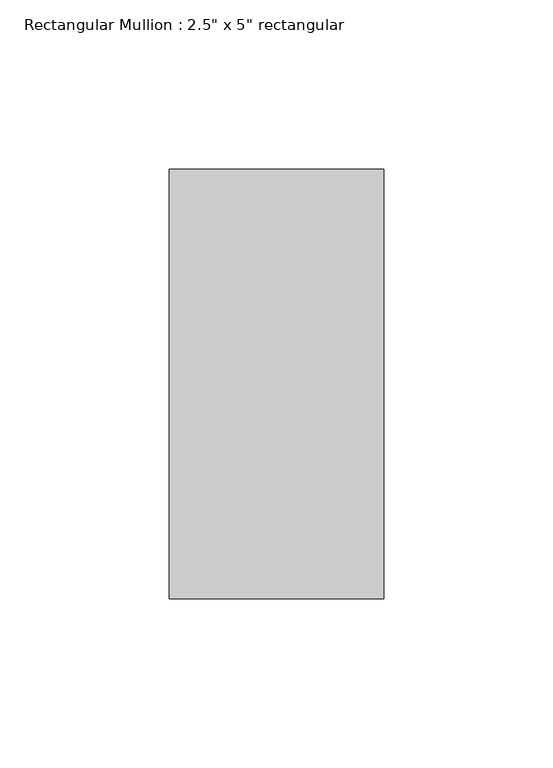
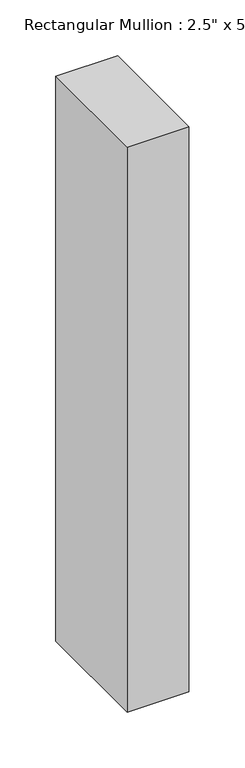
"""IFC4 building model written with IfcOpenShell, lengths in millimetres: member geometry."""

from ifc_helpers import new_model, si_unit, frame, origin, place, context, project, spatial, polyline, outline, extrude, source, transform, mapped, element, save


def member_3f0e0172(model_context):
    return source(origin(), model_context, "Body", "SweptSolid", [
        extrude(outline(polyline([(0.0, 63.5), (0.0, -63.5), (-63.5, -63.5), (-63.5, 63.5), (0.0, 63.5)])), frame((0.0, 0.0, -615.95), z_axis=(0.0, 0.0, 1.0), x_axis=(1.0, 0.0, 0.0)), (0.0, 0.0, 1.0), 615.95),
    ])


if __name__ == "__main__":
    model = new_model("IFC4")
    model_context = context("Model", 3, world=origin())
    ifc_project = project(units=[si_unit("LENGTHUNIT", "METRE", prefix="MILLI")], contexts=[model_context])
    site = spatial("IfcSite", under=ifc_project)
    building = spatial("IfcBuilding", under=site)
    placement = place(None, origin())
    member_shape = member_3f0e0172(model_context)
    element("IfcMember", 1, ObjectType="Rectangular Mullion : 2.5\" x 5\" rectangular", at=placement, inside=building, context=model_context, shape_type="MappedRepresentation", body=[
        mapped(member_shape, transform((0.0, 0.0, 0.0), x_axis=(1.0, 0.0, 0.0), y_axis=(0.0, 1.0, 0.0), z_axis=(0.0, 0.0, 1.0))),
    ])
    save(model, "model.ifc")

# Revit data of these elements
# Type "Rectangular Mullion : 2.5\" x 5\" rectangular"
#   built-in parameter 1007304 = 0.416667 (stored number, unit not read)
#   built-in parameter 1007301 = 0.104167 (stored number, unit not read)
#   built-in parameter 1007300 = 0.104167 (stored number, unit not read)
